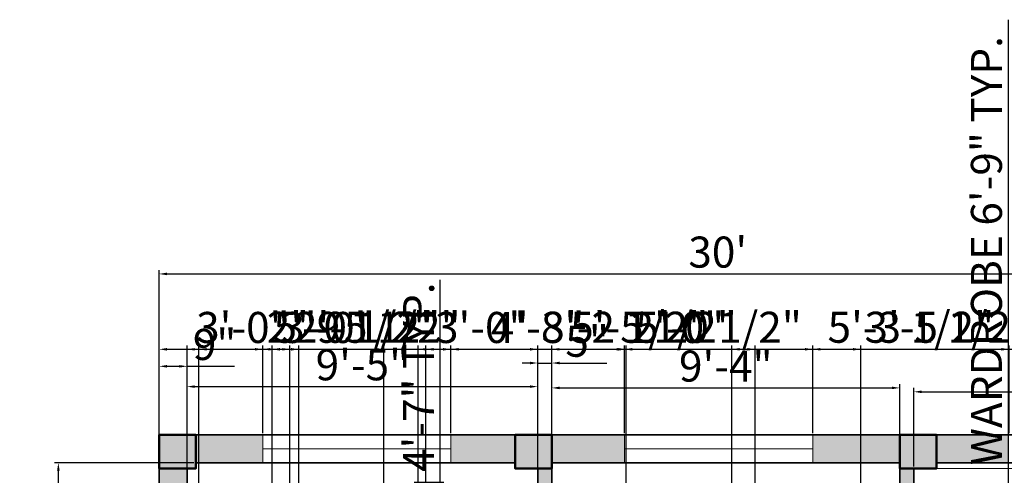
# Model space of a CAD drawing. Units: inches. Extents: x 2312 to 2808, y 1290 to 1909.
# Tile 4 of 5: x 2316 to 2633, y 1763 to 1909. Entities that reach past the tile are written whole.
import ezdxf

# ---------------------------------------------------------------- set-up
doc = ezdxf.new("R2010")
doc.units = ezdxf.units.IN
for name, color, linetype, lineweight in [('A-ANNO-DIMS', 2, 'Continuous', 18), ('A-COLS-PATT', 1, 'Continuous', 13), ('A-WALL-PATT', 150, 'Continuous', 13), ('COLUMN', 1, 'Continuous', 50), ('WALL', 7, 'Continuous', 35), ('WINDOW', 70, 'Continuous', 18)]:
    doc.layers.add(name, color=color, linetype=linetype, lineweight=lineweight)
doc.styles.get("Standard").update_dxf_attribs({"font": 'arial.ttf'})
doc.dimstyles.new('ISO-25', dxfattribs={"dimtxt": 10, "dimasz": 2.5, "dimexe": 1.25, "dimexo": 0.625, "dimtad": 1, "dimdec": 0, "dimlunit": 4, "dimtxsty": 'Standard', "dimcen": 2.5, "dimadec": 0, "dimazin": 0, "dimtfac": 1, "dimtdec": 0, "dimtmove": 0, "dimatfit": 3, "dimfxl": 1, "dimarcsym": 0})

# ---------------------------------------------------------------- blocks, each defined once
blk = doc.blocks.new('*D5')
at = {"layer": 'A-ANNO-DIMS', "color": 0, "lineweight": -2, "transparency": 16777216}
for p, q in [((2360.43, 1776.34), (2360.43, 1828.83)), ((2362.93, 1827.58), (2717.93, 1827.58)), ((2720.43, 1776.34), (2720.43, 1828.83))]:
    blk.add_line(p, q, dxfattribs=at)
at = {"layer": 'A-ANNO-DIMS', "color": 0, "transparency": 16777216}
for points in [[(2362.93, 1828), (2362.93, 1827.17), (2360.43, 1827.58)], [(2717.93, 1828), (2717.93, 1827.17), (2720.43, 1827.58)]]:
    blk.add_solid(points, dxfattribs=at)
at = {"layer": 'Defpoints', "color": 0, "transparency": 16777216}
for p in [(2720.43, 1827.58), (2360.43, 1775.72), (2720.43, 1775.72)]:
    blk.add_point(p, dxfattribs=at)
at = {"layer": 'A-ANNO-DIMS', "color": 0, "transparency": 16777216, "insert": (2540.43, 1833.32), "char_height": 10, "attachment_point": 5}
blk.add_mtext("30'", dxfattribs=at)
blk = doc.blocks.new('*D7')
at = {"layer": 'A-ANNO-DIMS', "color": 0, "lineweight": -2, "transparency": 16777216}
for p, q in [((2369.43, 1765.57), (2369.43, 1792.55)), ((2482.43, 1765.57), (2482.43, 1792.55)), ((2371.93, 1791.3), (2479.93, 1791.3))]:
    blk.add_line(p, q, dxfattribs=at)
at = {"layer": 'A-ANNO-DIMS', "color": 0, "transparency": 16777216}
for points in [[(2371.93, 1791.72), (2371.93, 1790.88), (2369.43, 1791.3)], [(2479.93, 1791.72), (2479.93, 1790.88), (2482.43, 1791.3)]]:
    blk.add_solid(points, dxfattribs=at)
at = {"layer": 'Defpoints', "color": 0, "transparency": 16777216}
for p in [(2482.43, 1791.3), (2369.43, 1764.94), (2482.43, 1764.94)]:
    blk.add_point(p, dxfattribs=at)
at = {"layer": 'A-ANNO-DIMS', "color": 0, "transparency": 16777216, "insert": (2425.93, 1797.03), "char_height": 10, "attachment_point": 5}
blk.add_mtext('9\'-5"', dxfattribs=at)
blk = doc.blocks.new('*D8')
at = {"layer": 'A-ANNO-DIMS', "color": 0, "lineweight": -2, "transparency": 16777216}
for p, q in [((2360.43, 1765.57), (2360.43, 1799.09)), ((2369.43, 1765.57), (2369.43, 1799.09)), ((2362.93, 1797.84), (2366.93, 1797.84)), ((2369.43, 1797.84), (2384.68, 1797.84))]:
    blk.add_line(p, q, dxfattribs=at)
at = {"layer": 'A-ANNO-DIMS', "color": 0, "transparency": 16777216}
for points in [[(2362.93, 1798.25), (2362.93, 1797.42), (2360.43, 1797.84)], [(2366.93, 1798.25), (2366.93, 1797.42), (2369.43, 1797.84)]]:
    blk.add_solid(points, dxfattribs=at)
at = {"layer": 'Defpoints', "color": 0, "transparency": 16777216}
for p in [(2369.43, 1797.84), (2360.43, 1764.94), (2369.43, 1764.94)]:
    blk.add_point(p, dxfattribs=at)
at = {"layer": 'A-ANNO-DIMS', "color": 0, "transparency": 16777216, "insert": (2378.31, 1803.57), "char_height": 10, "attachment_point": 5}
blk.add_mtext('9"', dxfattribs=at)
blk = doc.blocks.new('*D9')
at = {"layer": 'A-ANNO-DIMS', "color": 0, "lineweight": -2, "transparency": 16777216}
for p, q in [((2479.93, 1798.9), (2477.43, 1798.9)), ((2482.43, 1765.57), (2482.43, 1800.15)), ((2482.43, 1798.9), (2486.97, 1798.9)), ((2486.97, 1765.57), (2486.97, 1800.15)), ((2489.47, 1798.9), (2504.71, 1798.9))]:
    blk.add_line(p, q, dxfattribs=at)
at = {"layer": 'A-ANNO-DIMS', "color": 0, "transparency": 16777216}
for points in [[(2479.93, 1799.32), (2479.93, 1798.48), (2482.43, 1798.9)], [(2489.47, 1799.32), (2489.47, 1798.48), (2486.97, 1798.9)]]:
    blk.add_solid(points, dxfattribs=at)
at = {"layer": 'Defpoints', "color": 0, "transparency": 16777216}
for p in [(2486.97, 1798.9), (2482.43, 1764.94), (2486.97, 1764.94)]:
    blk.add_point(p, dxfattribs=at)
at = {"layer": 'A-ANNO-DIMS', "color": 0, "transparency": 16777216, "insert": (2498.34, 1804.61), "char_height": 10, "attachment_point": 5}
blk.add_mtext('5"', dxfattribs=at)
blk = doc.blocks.new('*D10')
at = {"layer": 'A-ANNO-DIMS', "color": 0, "lineweight": -2, "transparency": 16777216}
for p, q in [((2486.97, 1765.57), (2486.97, 1792.13)), ((2489.47, 1790.88), (2596.57, 1790.88)), ((2599.07, 1765.57), (2599.07, 1792.13))]:
    blk.add_line(p, q, dxfattribs=at)
at = {"layer": 'A-ANNO-DIMS', "color": 0, "transparency": 16777216}
for points in [[(2489.47, 1791.3), (2489.47, 1790.47), (2486.97, 1790.88)], [(2596.57, 1791.3), (2596.57, 1790.47), (2599.07, 1790.88)]]:
    blk.add_solid(points, dxfattribs=at)
at = {"layer": 'Defpoints', "color": 0, "transparency": 16777216}
for p in [(2599.07, 1790.88), (2486.97, 1764.94), (2599.07, 1764.94)]:
    blk.add_point(p, dxfattribs=at)
at = {"layer": 'A-ANNO-DIMS', "color": 0, "transparency": 16777216, "insert": (2543.02, 1796.61), "char_height": 10, "attachment_point": 5}
blk.add_mtext('9\'-4"', dxfattribs=at)
blk = doc.blocks.new('*D11')
at = {"layer": 'A-ANNO-DIMS', "color": 0, "lineweight": -2, "transparency": 16777216}
for p, q in [((2603.61, 1765.57), (2603.61, 1790.88)), ((2606.11, 1789.63), (2708.93, 1789.63)), ((2711.43, 1765.57), (2711.43, 1790.88))]:
    blk.add_line(p, q, dxfattribs=at)
at = {"layer": 'A-ANNO-DIMS', "color": 0, "transparency": 16777216}
for points in [[(2606.11, 1790.04), (2606.11, 1789.21), (2603.61, 1789.63)], [(2708.93, 1790.04), (2708.93, 1789.21), (2711.43, 1789.63)]]:
    blk.add_solid(points, dxfattribs=at)
at = {"layer": 'Defpoints', "color": 0, "transparency": 16777216}
for p in [(2711.43, 1789.63), (2603.61, 1764.94), (2711.43, 1764.94)]:
    blk.add_point(p, dxfattribs=at)
at = {"layer": 'A-ANNO-DIMS', "color": 0, "transparency": 16777216, "insert": (2657.52, 1795.36), "char_height": 10, "attachment_point": 5}
blk.add_mtext("9'", dxfattribs=at)
blk = doc.blocks.new('*D12')
at = {"layer": 'A-ANNO-DIMS', "color": 0, "lineweight": -2, "transparency": 16777216}
for p, q in [((2604.24, 1764.94), (2740.72, 1765.28)), ((2739.79, 1637.55), (2739.48, 1762.78)), ((2604.56, 1634.72), (2741.04, 1635.06))]:
    blk.add_line(p, q, dxfattribs=at)
at = {"layer": 'A-ANNO-DIMS', "color": 0, "transparency": 16777216}
for points in [[(2739.89, 1762.78), (2739.06, 1762.78), (2739.47, 1765.28)], [(2740.2, 1637.56), (2739.37, 1637.55), (2739.79, 1635.05)]]:
    blk.add_solid(points, dxfattribs=at)
at = {"layer": 'Defpoints', "color": 0, "transparency": 16777216}
for p in [(2603.61, 1764.94), (2739.47, 1765.28), (2603.93, 1634.72)]:
    blk.add_point(p, dxfattribs=at)
at = {"layer": 'A-ANNO-DIMS', "color": 0, "transparency": 16777216, "insert": (2745.36, 1700.18), "char_height": 10, "attachment_point": 5, "rotation": 270.1423}
blk.add_mtext('10\'-10"', dxfattribs=at)
blk = doc.blocks.new('*D21')
at = {"layer": 'A-ANNO-DIMS', "color": 0, "lineweight": -2, "transparency": 16777216}
for p, q in [((2371.65, 1766.72), (2326.71, 1766.72)), ((2327.96, 1637.22), (2327.96, 1764.22)), ((2371.65, 1634.72), (2326.71, 1634.72))]:
    blk.add_line(p, q, dxfattribs=at)
at = {"layer": 'A-ANNO-DIMS', "color": 0, "transparency": 16777216}
for points in [[(2327.54, 1764.22), (2328.38, 1764.22), (2327.96, 1766.72)], [(2327.54, 1637.22), (2328.38, 1637.22), (2327.96, 1634.72)]]:
    blk.add_solid(points, dxfattribs=at)
at = {"layer": 'Defpoints', "color": 0, "transparency": 16777216}
for p in [(2327.96, 1766.72), (2372.28, 1766.72), (2372.28, 1634.72)]:
    blk.add_point(p, dxfattribs=at)
at = {"layer": 'A-ANNO-DIMS', "color": 0, "transparency": 16777216, "insert": (2322.31, 1700.72), "char_height": 10, "attachment_point": 5, "rotation": 90}
blk.add_mtext("11'", dxfattribs=at)
blk = doc.blocks.new('*D30')
at = {"layer": 'A-ANNO-DIMS', "color": 0, "lineweight": -2, "transparency": 16777216}
for p, q in [((2450.95, 1760.54), (2450.95, 1825.65)), ((2442.63, 1760.54), (2452.2, 1760.54)), ((2450.95, 1707.96), (2450.95, 1758.04)), ((2442.63, 1705.46), (2452.2, 1705.46))]:
    blk.add_line(p, q, dxfattribs=at)
at = {"layer": 'A-ANNO-DIMS', "color": 0, "transparency": 16777216}
for points in [[(2450.54, 1758.04), (2451.37, 1758.04), (2450.95, 1760.54)], [(2450.54, 1707.96), (2451.37, 1707.96), (2450.95, 1705.46)]]:
    blk.add_solid(points, dxfattribs=at)
at = {"layer": 'Defpoints', "color": 0, "transparency": 16777216}
for p in [(2442, 1760.54), (2450.95, 1760.54), (2442, 1705.46)]:
    blk.add_point(p, dxfattribs=at)
at = {"layer": 'A-ANNO-DIMS', "color": 0, "transparency": 16777216, "insert": (2445.32, 1794.34), "char_height": 10, "attachment_point": 5, "rotation": 90}
blk.add_mtext('4\'-7" TYP.', dxfattribs=at)
blk = doc.blocks.new('*D31')
at = {"layer": 'A-ANNO-DIMS', "color": 0, "lineweight": -2, "transparency": 16777216}
for p, q in [((2634.1, 1758.19), (2634.1, 1909.46)), ((2622.58, 1758.19), (2635.35, 1758.19)), ((2634.1, 1679.72), (2634.1, 1755.69)), ((2622.58, 1677.22), (2635.35, 1677.22))]:
    blk.add_line(p, q, dxfattribs=at)
at = {"layer": 'A-ANNO-DIMS', "color": 0, "transparency": 16777216}
for points in [[(2633.68, 1755.69), (2634.51, 1755.69), (2634.1, 1758.19)], [(2633.68, 1679.72), (2634.51, 1679.72), (2634.1, 1677.22)]]:
    blk.add_solid(points, dxfattribs=at)
at = {"layer": 'Defpoints', "color": 0, "transparency": 16777216}
for p in [(2621.95, 1758.19), (2634.1, 1758.19), (2621.95, 1677.22)]:
    blk.add_point(p, dxfattribs=at)
at = {"layer": 'A-ANNO-DIMS', "color": 0, "transparency": 16777216, "insert": (2628.3, 1835.07), "char_height": 10, "attachment_point": 5, "rotation": 90}
blk.add_mtext('WARDROBE 6\'-9" TYP.', dxfattribs=at)
blk = doc.blocks.new('*D41')
at = {"layer": 'A-ANNO-DIMS', "color": 0, "lineweight": -2, "transparency": 16777216}
for p, q in [((2443.93, 1546.83), (2443.93, 1804.57)), ((2446.43, 1803.32), (2479.93, 1803.32)), ((2482.43, 1510.12), (2482.43, 1804.57)), ((2482.43, 1803.32), (2536.06, 1803.32))]:
    blk.add_line(p, q, dxfattribs=at)
at = {"layer": 'A-ANNO-DIMS', "color": 0, "transparency": 16777216}
for points in [[(2446.43, 1803.73), (2446.43, 1802.9), (2443.93, 1803.32)], [(2479.93, 1803.73), (2479.93, 1802.9), (2482.43, 1803.32)]]:
    blk.add_solid(points, dxfattribs=at)
at = {"layer": 'Defpoints', "color": 0, "transparency": 16777216}
for p in [(2482.43, 1803.32), (2443.93, 1546.2), (2482.43, 1509.49)]:
    blk.add_point(p, dxfattribs=at)
at = {"layer": 'A-ANNO-DIMS', "color": 0, "transparency": 16777216, "insert": (2510.5, 1809.12), "char_height": 10, "attachment_point": 5}
blk.add_mtext('3\'-2 1/2"', dxfattribs=at)
blk = doc.blocks.new('*D43')
at = {"layer": 'A-ANNO-DIMS', "color": 0, "lineweight": -2, "transparency": 16777216}
for p, q in [((2486.93, 1401.34), (2486.93, 1804.57)), ((2489.43, 1803.32), (2508.43, 1803.32)), ((2510.93, 1401.34), (2510.93, 1804.57)), ((2510.93, 1803.32), (2541.44, 1803.32))]:
    blk.add_line(p, q, dxfattribs=at)
at = {"layer": 'A-ANNO-DIMS', "color": 0, "transparency": 16777216}
for points in [[(2489.43, 1803.73), (2489.43, 1802.9), (2486.93, 1803.32)], [(2508.43, 1803.73), (2508.43, 1802.9), (2510.93, 1803.32)]]:
    blk.add_solid(points, dxfattribs=at)
at = {"layer": 'Defpoints', "color": 0, "transparency": 16777216}
for p in [(2510.93, 1803.32), (2486.93, 1400.72), (2510.93, 1400.72)]:
    blk.add_point(p, dxfattribs=at)
at = {"layer": 'A-ANNO-DIMS', "color": 0, "transparency": 16777216, "insert": (2527.44, 1809.05), "char_height": 10, "attachment_point": 5}
blk.add_mtext('2\'-0"', dxfattribs=at)
blk = doc.blocks.new('*D44')
at = {"layer": 'A-ANNO-DIMS', "color": 0, "lineweight": -2, "transparency": 16777216}
for p, q in [((2360.43, 1776.34), (2360.43, 1804.57)), ((2362.93, 1803.32), (2391.3, 1803.32)), ((2393.8, 1776.34), (2393.8, 1804.57)), ((2393.8, 1803.32), (2447.6, 1803.32))]:
    blk.add_line(p, q, dxfattribs=at)
at = {"layer": 'A-ANNO-DIMS', "color": 0, "transparency": 16777216}
for points in [[(2362.93, 1803.73), (2362.93, 1802.9), (2360.43, 1803.32)], [(2391.3, 1803.73), (2391.3, 1802.9), (2393.8, 1803.32)]]:
    blk.add_solid(points, dxfattribs=at)
at = {"layer": 'Defpoints', "color": 0, "transparency": 16777216}
for p in [(2393.8, 1803.32), (2360.43, 1775.72), (2393.8, 1775.72)]:
    blk.add_point(p, dxfattribs=at)
at = {"layer": 'A-ANNO-DIMS', "color": 0, "transparency": 16777216, "insert": (2421.95, 1809.11), "char_height": 10, "attachment_point": 5}
blk.add_mtext('2\'-9 1/2"', dxfattribs=at)
blk = doc.blocks.new('*D45')
at = {"layer": 'A-ANNO-DIMS', "color": 0, "lineweight": -2, "transparency": 16777216}
for p, q in [((2393.8, 1776.34), (2393.8, 1804.57)), ((2396.3, 1803.32), (2451.95, 1803.32)), ((2454.45, 1776.34), (2454.45, 1804.57))]:
    blk.add_line(p, q, dxfattribs=at)
at = {"layer": 'A-ANNO-DIMS', "color": 0, "transparency": 16777216}
for points in [[(2396.3, 1803.73), (2396.3, 1802.9), (2393.8, 1803.32)], [(2451.95, 1803.73), (2451.95, 1802.9), (2454.45, 1803.32)]]:
    blk.add_solid(points, dxfattribs=at)
at = {"layer": 'Defpoints', "color": 0, "transparency": 16777216}
for p in [(2454.45, 1803.32), (2393.8, 1775.72), (2454.45, 1775.72)]:
    blk.add_point(p, dxfattribs=at)
at = {"layer": 'A-ANNO-DIMS', "color": 0, "transparency": 16777216, "insert": (2424.12, 1809.11), "char_height": 10, "attachment_point": 5}
blk.add_mtext('5\'-0 1/2"', dxfattribs=at)
blk = doc.blocks.new('*D46')
at = {"layer": 'A-ANNO-DIMS', "color": 0, "lineweight": -2, "transparency": 16777216}
for p, q in [((2454.45, 1776.34), (2454.45, 1804.57)), ((2456.95, 1803.32), (2507.86, 1803.32)), ((2510.36, 1776.34), (2510.36, 1804.57))]:
    blk.add_line(p, q, dxfattribs=at)
at = {"layer": 'A-ANNO-DIMS', "color": 0, "transparency": 16777216}
for points in [[(2456.95, 1803.73), (2456.95, 1802.9), (2454.45, 1803.32)], [(2507.86, 1803.73), (2507.86, 1802.9), (2510.36, 1803.32)]]:
    blk.add_solid(points, dxfattribs=at)
at = {"layer": 'Defpoints', "color": 0, "transparency": 16777216}
for p in [(2510.36, 1803.32), (2454.45, 1775.72), (2510.36, 1775.72)]:
    blk.add_point(p, dxfattribs=at)
at = {"layer": 'A-ANNO-DIMS', "color": 0, "transparency": 16777216, "insert": (2482.41, 1809.05), "char_height": 10, "attachment_point": 5}
blk.add_mtext('4\'-8"', dxfattribs=at)
blk = doc.blocks.new('*D47')
at = {"layer": 'A-ANNO-DIMS', "color": 0, "lineweight": -2, "transparency": 16777216}
for p, q in [((2510.36, 1776.34), (2510.36, 1804.57)), ((2512.86, 1803.32), (2568.52, 1803.32)), ((2571.02, 1776.34), (2571.02, 1804.57))]:
    blk.add_line(p, q, dxfattribs=at)
at = {"layer": 'A-ANNO-DIMS', "color": 0, "transparency": 16777216}
for points in [[(2512.86, 1803.73), (2512.86, 1802.9), (2510.36, 1803.32)], [(2568.52, 1803.73), (2568.52, 1802.9), (2571.02, 1803.32)]]:
    blk.add_solid(points, dxfattribs=at)
at = {"layer": 'Defpoints', "color": 0, "transparency": 16777216}
for p in [(2571.02, 1803.32), (2510.36, 1775.72), (2571.02, 1775.72)]:
    blk.add_point(p, dxfattribs=at)
at = {"layer": 'A-ANNO-DIMS', "color": 0, "transparency": 16777216, "insert": (2540.69, 1809.11), "char_height": 10, "attachment_point": 5}
blk.add_mtext('5\'-0 1/2"', dxfattribs=at)
blk = doc.blocks.new('*D48')
at = {"layer": 'A-ANNO-DIMS', "color": 0, "lineweight": -2, "transparency": 16777216}
for p, q in [((2571.02, 1776.34), (2571.02, 1804.57)), ((2573.52, 1803.32), (2631.81, 1803.32)), ((2634.31, 1776.34), (2634.31, 1804.57))]:
    blk.add_line(p, q, dxfattribs=at)
at = {"layer": 'A-ANNO-DIMS', "color": 0, "transparency": 16777216}
for points in [[(2573.52, 1803.73), (2573.52, 1802.9), (2571.02, 1803.32)], [(2631.81, 1803.73), (2631.81, 1802.9), (2634.31, 1803.32)]]:
    blk.add_solid(points, dxfattribs=at)
at = {"layer": 'Defpoints', "color": 0, "transparency": 16777216}
for p in [(2634.31, 1803.32), (2571.02, 1775.72), (2634.31, 1775.72)]:
    blk.add_point(p, dxfattribs=at)
at = {"layer": 'A-ANNO-DIMS', "color": 0, "transparency": 16777216, "insert": (2602.66, 1809.12), "char_height": 10, "attachment_point": 5}
blk.add_mtext('5\'-3 1/2"', dxfattribs=at)
blk = doc.blocks.new('*D50')
at = {"layer": 'A-ANNO-DIMS', "color": 0, "lineweight": -2, "transparency": 16777216}
for p, q in [((2446.36, 1635.34), (2446.36, 1804.57)), ((2448.86, 1803.32), (2479.93, 1803.32)), ((2482.43, 1635.34), (2482.43, 1804.57))]:
    blk.add_line(p, q, dxfattribs=at)
at = {"layer": 'A-ANNO-DIMS', "color": 0, "transparency": 16777216}
for points in [[(2448.86, 1803.73), (2448.86, 1802.9), (2446.36, 1803.32)], [(2479.93, 1803.73), (2479.93, 1802.9), (2482.43, 1803.32)]]:
    blk.add_solid(points, dxfattribs=at)
at = {"layer": 'Defpoints', "color": 0, "transparency": 16777216}
for p in [(2482.43, 1803.32), (2446.36, 1634.72), (2482.43, 1634.72)]:
    blk.add_point(p, dxfattribs=at)
at = {"layer": 'A-ANNO-DIMS', "color": 0, "transparency": 16777216, "insert": (2464.4, 1809.05), "char_height": 10, "attachment_point": 5}
blk.add_mtext('3\'-0"', dxfattribs=at)
blk = doc.blocks.new('*D53')
at = {"layer": 'A-ANNO-DIMS', "color": 0, "lineweight": -2, "transparency": 16777216}
for p, q in [((2369.43, 1543.69), (2369.43, 1804.57)), ((2371.93, 1803.32), (2402.93, 1803.32)), ((2405.43, 1539.84), (2405.43, 1804.57))]:
    blk.add_line(p, q, dxfattribs=at)
at = {"layer": 'A-ANNO-DIMS', "color": 0, "transparency": 16777216}
for points in [[(2371.93, 1803.73), (2371.93, 1802.9), (2369.43, 1803.32)], [(2402.93, 1803.73), (2402.93, 1802.9), (2405.43, 1803.32)]]:
    blk.add_solid(points, dxfattribs=at)
at = {"layer": 'Defpoints', "color": 0, "transparency": 16777216}
for p in [(2405.43, 1803.32), (2369.43, 1543.07), (2405.43, 1539.22)]:
    blk.add_point(p, dxfattribs=at)
at = {"layer": 'A-ANNO-DIMS', "color": 0, "transparency": 16777216, "insert": (2387.43, 1809.05), "char_height": 10, "attachment_point": 5}
blk.add_mtext('3\'-0"', dxfattribs=at)
blk = doc.blocks.new('*D54')
at = {"layer": 'A-ANNO-DIMS', "color": 0, "lineweight": -2, "transparency": 16777216}
for p, q in [((2545.01, 1581.25), (2545.01, 1804.57)), ((2547.51, 1803.32), (2583.99, 1803.32)), ((2586.49, 1581.25), (2586.49, 1804.57)), ((2586.49, 1803.32), (2640.12, 1803.32))]:
    blk.add_line(p, q, dxfattribs=at)
at = {"layer": 'A-ANNO-DIMS', "color": 0, "transparency": 16777216}
for points in [[(2547.51, 1803.73), (2547.51, 1802.9), (2545.01, 1803.32)], [(2583.99, 1803.73), (2583.99, 1802.9), (2586.49, 1803.32)]]:
    blk.add_solid(points, dxfattribs=at)
at = {"layer": 'Defpoints', "color": 0, "transparency": 16777216}
for p in [(2586.49, 1803.32), (2545.01, 1580.62), (2586.49, 1580.62)]:
    blk.add_point(p, dxfattribs=at)
at = {"layer": 'A-ANNO-DIMS', "color": 0, "transparency": 16777216, "insert": (2614.56, 1809.12), "char_height": 10, "attachment_point": 5}
blk.add_mtext('3\'-5 1/2"', dxfattribs=at)
blk = doc.blocks.new('*D62')
at = {"layer": 'A-ANNO-DIMS', "color": 0, "lineweight": -2, "transparency": 16777216}
for p, q in [((2396.83, 1508.42), (2396.83, 1804.57)), ((2399.33, 1803.32), (2430.33, 1803.32)), ((2432.83, 1508.42), (2432.83, 1804.57))]:
    blk.add_line(p, q, dxfattribs=at)
at = {"layer": 'A-ANNO-DIMS', "color": 0, "transparency": 16777216}
for points in [[(2399.33, 1803.73), (2399.33, 1802.9), (2396.83, 1803.32)], [(2430.33, 1803.73), (2430.33, 1802.9), (2432.83, 1803.32)]]:
    blk.add_solid(points, dxfattribs=at)
at = {"layer": 'Defpoints', "color": 0, "transparency": 16777216}
for p in [(2432.83, 1803.32), (2396.83, 1507.8), (2432.83, 1507.8)]:
    blk.add_point(p, dxfattribs=at)
at = {"layer": 'A-ANNO-DIMS', "color": 0, "transparency": 16777216, "insert": (2414.83, 1809.05), "char_height": 10, "attachment_point": 5}
blk.add_mtext('3\'-0"', dxfattribs=at)
blk = doc.blocks.new('*D67')
at = {"layer": 'A-ANNO-DIMS', "color": 0, "lineweight": -2, "transparency": 16777216}
for p, q in [((2486.93, 1499.34), (2486.93, 1804.57)), ((2489.43, 1803.32), (2550.01, 1803.32)), ((2552.51, 1499.34), (2552.51, 1804.57))]:
    blk.add_line(p, q, dxfattribs=at)
at = {"layer": 'A-ANNO-DIMS', "color": 0, "transparency": 16777216}
for points in [[(2489.43, 1803.73), (2489.43, 1802.9), (2486.93, 1803.32)], [(2550.01, 1803.73), (2550.01, 1802.9), (2552.51, 1803.32)]]:
    blk.add_solid(points, dxfattribs=at)
at = {"layer": 'Defpoints', "color": 0, "transparency": 16777216}
for p in [(2552.51, 1803.32), (2486.93, 1498.72), (2552.51, 1498.72)]:
    blk.add_point(p, dxfattribs=at)
at = {"layer": 'A-ANNO-DIMS', "color": 0, "transparency": 16777216, "insert": (2519.72, 1809.11), "char_height": 10, "attachment_point": 5}
blk.add_mtext('5\'-5 1/2"', dxfattribs=at)
blk = doc.blocks.new('*D73')
at = {"layer": 'A-ANNO-DIMS', "color": 0, "lineweight": -2, "transparency": 16777216}
for p, q in [((2373.27, 1609.07), (2373.27, 1804.57)), ((2375.77, 1803.32), (2400.08, 1803.32)), ((2402.58, 1609.07), (2402.58, 1804.57)), ((2402.58, 1803.32), (2456.39, 1803.32))]:
    blk.add_line(p, q, dxfattribs=at)
at = {"layer": 'A-ANNO-DIMS', "color": 0, "transparency": 16777216}
for points in [[(2375.77, 1803.73), (2375.77, 1802.9), (2373.27, 1803.32)], [(2400.08, 1803.73), (2400.08, 1802.9), (2402.58, 1803.32)]]:
    blk.add_solid(points, dxfattribs=at)
at = {"layer": 'Defpoints', "color": 0, "transparency": 16777216}
for p in [(2402.58, 1803.32), (2373.27, 1608.44), (2402.58, 1608.44)]:
    blk.add_point(p, dxfattribs=at)
at = {"layer": 'A-ANNO-DIMS', "color": 0, "transparency": 16777216, "insert": (2430.74, 1809.11), "char_height": 10, "attachment_point": 5}
blk.add_mtext('2\'-5 1/2"', dxfattribs=at)

msp = doc.modelspace()

# ---------------------------------------------------------------- hatches: boundary and pattern name
at = {"layer": 'A-COLS-PATT'}
h = msp.add_hatch(color=256, dxfattribs=at)
h.dxf.hatch_style = 1
h.paths.add_polyline_path([(2372.28, 1775.72), (2360.43, 1775.72), (2360.43, 1764.94), (2372.28, 1764.94)])
h.paths.add_polyline_path([(2486.97, 1775.72), (2475.12, 1775.72), (2475.12, 1764.94), (2486.93, 1764.94), (2486.93, 1766.72)])
h.paths.add_polyline_path([(2610.92, 1775.72), (2599.07, 1775.72), (2599.07, 1766.72), (2599.11, 1766.72), (2599.11, 1764.94), (2610.92, 1764.94)])
h.paths.add_polyline_path([(2720.43, 1775.72), (2708.59, 1775.72), (2708.59, 1764.94), (2720.43, 1764.94)])
h.paths.add_polyline_path([(2723.28, 1640.11), (2711.43, 1640.11), (2711.43, 1629.34), (2723.28, 1629.34)])
h.paths.add_polyline_path([(2603.61, 1640.99), (2592.09, 1640.99), (2592.09, 1630.22), (2603.93, 1630.22), (2603.93, 1634.72), (2603.61, 1634.72)])
h.paths.add_polyline_path([(2494.28, 1640.99), (2482.43, 1640.99), (2482.43, 1630.22), (2494.28, 1630.22)])
h.paths.add_polyline_path([(2372.28, 1640.99), (2360.43, 1640.99), (2360.43, 1630.22), (2372.28, 1630.22)])
h.paths.add_polyline_path([(2372.28, 1509.49), (2360.43, 1509.49), (2360.43, 1498.72), (2372.28, 1498.72)])
h.paths.add_polyline_path([(2494.28, 1509.49), (2482.43, 1509.49), (2482.43, 1498.72), (2494.28, 1498.72)])
h.paths.add_polyline_path([(2603.93, 1509.49), (2592.09, 1509.49), (2592.09, 1498.72), (2603.93, 1498.72)])
h.paths.add_polyline_path([(2723.28, 1509.26), (2711.43, 1509.26), (2711.43, 1498.48), (2723.28, 1498.48)])
h.paths.add_polyline_path([(2720.43, 1378.49), (2708.59, 1378.49), (2708.59, 1367.72), (2720.43, 1367.72)])
h.paths.add_polyline_path([(2610.2, 1378.49), (2598.36, 1378.49), (2598.36, 1367.72), (2610.2, 1367.72)])
h.paths.add_polyline_path([(2486.94, 1376.72), (2486.93, 1376.72), (2486.93, 1378.49), (2475.1, 1378.49), (2475.1, 1367.72), (2486.94, 1367.72)])
h.paths.add_polyline_path([(2372.28, 1378.49), (2360.43, 1378.49), (2360.43, 1367.72), (2372.28, 1367.72)])
at = {"layer": 'A-WALL-PATT'}
h = msp.add_hatch(color=256, dxfattribs=at)
h.dxf.hatch_style = 1
h.paths.add_polyline_path([(2369.43, 1764.94), (2360.43, 1764.94), (2360.43, 1640.99), (2369.43, 1640.99)])
h.paths.add_polyline_path([(2720.43, 1764.94), (2711.43, 1764.94), (2711.43, 1640.11), (2720.43, 1640.11)])
h.paths.add_polyline_path([(2552.09, 1634.72), (2494.28, 1634.72), (2494.28, 1630.22), (2552.09, 1630.22)])
h.paths.add_polyline_path([(2446.36, 1634.72), (2372.28, 1634.72), (2372.28, 1630.22), (2405.43, 1630.22), (2439.43, 1630.22), (2446.36, 1630.22)])
h.paths.add_polyline_path([(2443.93, 1630.22), (2439.43, 1630.22), (2439.43, 1596.05), (2443.93, 1596.05)])
h.paths.add_polyline_path([(2486.93, 1630.22), (2482.43, 1630.22), (2482.43, 1509.49), (2486.93, 1509.49)])
h.paths.add_polyline_path([(2443.93, 1546.2), (2439.43, 1546.2), (2439.43, 1503.22), (2372.28, 1503.22), (2372.28, 1498.72), (2443.93, 1498.72)])
h.paths.add_polyline_path([(2555.45, 1503.22), (2494.28, 1503.22), (2494.28, 1498.72), (2555.45, 1498.72)])
h.paths.add_polyline_path([(2711.43, 1503.22), (2639.88, 1503.22), (2639.88, 1498.72), (2711.43, 1498.72)])
h.paths.add_polyline_path([(2646.41, 1564.72), (2711.43, 1564.72), (2711.43, 1569.22), (2646.41, 1569.22), (2646.41, 1597.21), (2641.91, 1597.21), (2641.91, 1564.72), (2641.91, 1536.48), (2646.41, 1536.48)])
h.paths.add_polyline_path([(2720.43, 1498.48), (2711.43, 1498.48), (2711.43, 1378.49), (2720.43, 1378.49)])
h.paths.add_polyline_path([(2369.43, 1498.72), (2360.43, 1498.72), (2360.43, 1378.49), (2369.43, 1378.49)])
h.paths.add_polyline_path([(2486.93, 1498.72), (2482.43, 1498.72), (2482.43, 1378.49), (2486.93, 1378.49)])
h.paths.add_polyline_path([(2603.93, 1498.72), (2599.11, 1498.72), (2599.11, 1378.49), (2603.93, 1378.49)])
h.paths.add_polyline_path([(2510.36, 1766.72), (2510.36, 1775.72), (2486.97, 1775.72), (2486.97, 1766.72)])
h.paths.add_polyline_path([(2571.02, 1775.72), (2571.02, 1766.72), (2599.07, 1766.72), (2599.07, 1775.72)])
h.paths.add_polyline_path([(2393.8, 1766.72), (2393.8, 1775.72), (2372.28, 1775.72), (2372.28, 1766.72)])
h.paths.add_polyline_path([(2454.45, 1775.72), (2454.45, 1766.72), (2475.12, 1766.72), (2475.12, 1775.72)])
h.paths.add_polyline_path([(2694.96, 1775.72), (2694.96, 1766.72), (2708.59, 1766.72), (2708.59, 1775.72)])
h.paths.add_polyline_path([(2634.31, 1766.72), (2634.31, 1775.72), (2610.92, 1775.72), (2610.92, 1766.72)])
h.paths.add_polyline_path([(2392.25, 1367.72), (2392.25, 1376.72), (2372.28, 1376.72), (2372.28, 1367.72)])
h.paths.add_polyline_path([(2452.9, 1376.72), (2452.9, 1367.72), (2475.1, 1367.72), (2475.1, 1376.72)])
h.paths.add_polyline_path([(2508.56, 1376.72), (2508.56, 1367.72), (2558.63, 1367.72), (2558.63, 1370.65), (2558.63, 1376.72)])
h.paths.add_polyline_path([(2488.96, 1367.72), (2488.96, 1376.72), (2486.94, 1376.72), (2486.94, 1367.72)])
h.paths.add_polyline_path([(2634.6, 1367.72), (2634.6, 1376.72), (2610.2, 1376.72), (2610.2, 1367.72)])
h.paths.add_polyline_path([(2695.25, 1376.72), (2695.25, 1367.72), (2708.59, 1367.72), (2708.59, 1376.72)])
h.paths.add_polyline_path([(2360.43, 1590.4), (2369.43, 1590.4), (2369.43, 1630.22), (2360.43, 1630.22)])
h.paths.add_polyline_path([(2369.43, 1543.07), (2360.43, 1543.07), (2360.43, 1509.49), (2369.43, 1509.49)])
h.paths.add_polyline_path([(2720.43, 1531.67), (2711.43, 1531.67), (2711.43, 1509.26), (2720.43, 1509.26)])
h.paths.add_polyline_path([(2720.43, 1572.68), (2711.43, 1572.68), (2711.43, 1558.71), (2720.43, 1558.71)])
h.paths.add_polyline_path([(2711.43, 1599.72), (2720.43, 1599.72), (2720.43, 1629.34), (2711.43, 1629.34)])
h = msp.add_hatch(color=256, dxfattribs=at)
h.dxf.hatch_style = 1
h.paths.add_polyline_path([(2486.93, 1764.94), (2482.43, 1764.94), (2482.43, 1640.99), (2486.93, 1640.99)])
h.paths.add_polyline_path([(2603.61, 1764.94), (2599.11, 1764.94), (2599.11, 1640.99), (2603.61, 1640.99)])

# ---------------------------------------------------------------- linework, layer by layer
at = {"layer": 'COLUMN'}
for points in [[(2360.43, 1775.72), (2372.28, 1775.72), (2372.28, 1764.94), (2360.43, 1764.94)], [(2475.12, 1775.72), (2486.97, 1775.72), (2486.97, 1764.94), (2475.12, 1764.94)], [(2599.07, 1775.72), (2610.92, 1775.72), (2610.92, 1764.94), (2599.07, 1764.94)]]:
    msp.add_lwpolyline(points, close=True, dxfattribs=at)
at = {"layer": 'WALL'}
for p, q in [((2360.43, 1775.72), (2720.43, 1775.72)), ((2360.43, 1367.72), (2360.43, 1775.72)), ((2372.28, 1766.72), (2475.12, 1766.72)), ((2482.43, 1764.94), (2482.43, 1634.72)), ((2486.93, 1766.72), (2486.93, 1640.99)), ((2486.93, 1766.72), (2599.11, 1766.72)), ((2599.11, 1766.72), (2599.11, 1640.99)), ((2603.61, 1764.94), (2603.61, 1634.72))]:
    msp.add_line(p, q, dxfattribs=at)
for points in [[(2720.43, 1498.48), (2720.43, 1367.72), (2360.43, 1367.72), (2360.43, 1775.72), (2720.43, 1775.72), (2720.43, 1640.11)], [(2369.43, 1640.99), (2369.43, 1764.94)], [(2372.28, 1766.72), (2475.12, 1766.72)], [(2486.93, 1766.72), (2599.11, 1766.72)], [(2610.92, 1766.72), (2708.59, 1766.72)]]:
    msp.add_lwpolyline(points, dxfattribs=at)
at = {"layer": 'WINDOW'}
for p, q in [((2393.8, 1771.22), (2454.45, 1771.22)), ((2510.36, 1771.22), (2571.02, 1771.22))]:
    msp.add_line(p, q, dxfattribs=at)
for points in [[(2393.8, 1775.72), (2454.45, 1775.72), (2454.45, 1766.72), (2393.8, 1766.72)], [(2510.36, 1775.72), (2571.02, 1775.72), (2571.02, 1766.72), (2510.36, 1766.72)]]:
    msp.add_lwpolyline(points, close=True, dxfattribs=at)

# ---------------------------------------------------------------- dimensions: what is measured, and where the dimension line sits
at = {"layer": 'A-ANNO-DIMS'}
for base, p1, p2, text, picture, middle in [((2634.1, 1758.19), (2621.95, 1677.22), (2621.95, 1758.19), 'WARDROBE <> TYP.', '*D31', (2628.3, 1835.07)), ((2450.95, 1760.54), (2442, 1705.46), (2442, 1760.54), '<> TYP.', '*D30', (2445.32, 1794.34))]:
    dim = msp.add_linear_dim(base=base, p1=p1, p2=p2, angle=90, text=text, dimstyle='ISO-25', override={"dimdec": 1, "dimlfac": 1, "dimrnd": 0, "dimzin": 1, "dimdsep": 46, "dimlunit": 4, "dimfrac": 2}, dxfattribs=at)
    dim.commit()
    dim.dimension.update_dxf_attribs({"geometry": picture, "text_midpoint": middle})
for base, p1, p2, override, picture, middle in [((2720.43, 1827.58), (2360.43, 1775.72), (2720.43, 1775.72), {"dimclrd": 0, "dimclre": 0, "dimclrt": 0}, '*D5', (2540.43, 1833.32)), ((2393.8, 1803.32), (2360.43, 1775.72), (2393.8, 1775.72), {"dimdec": 1, "dimlfac": 1, "dimrnd": 0, "dimzin": 1, "dimdsep": 46, "dimlunit": 4, "dimfrac": 2}, '*D44', (2421.95, 1809.11)), ((2402.58, 1803.32), (2373.27, 1608.44), (2402.58, 1608.44), {"dimdec": 1, "dimlfac": 1, "dimrnd": 0, "dimzin": 1, "dimdsep": 46, "dimlunit": 4, "dimfrac": 2}, '*D73', (2430.74, 1809.11)), ((2454.4493, 1803.3175), (2393.7969, 1775.7175), (2454.4493, 1775.7175), {"dimdec": 1, "dimlfac": 1, "dimrnd": 0, "dimzin": 1, "dimdsep": 46, "dimlunit": 4, "dimfrac": 2}, '*D45', (2424.1231, 1809.113)), ((2482.43, 1803.32), (2443.93, 1546.2), (2482.43, 1509.49), {"dimdec": 1, "dimlfac": 1, "dimrnd": 0, "dimzin": 1, "dimdsep": 46, "dimlunit": 4, "dimfrac": 2}, '*D41', (2510.5, 1809.12)), ((2552.51, 1803.32), (2486.93, 1498.72), (2552.51, 1498.72), {"dimdec": 1, "dimlfac": 1, "dimrnd": 0, "dimzin": 1, "dimdsep": 46, "dimlunit": 4, "dimfrac": 2}, '*D67', (2519.72, 1809.11)), ((2571.02, 1803.32), (2510.36, 1775.72), (2571.02, 1775.72), {"dimdec": 1, "dimlfac": 1, "dimrnd": 0, "dimzin": 1, "dimdsep": 46, "dimlunit": 4, "dimfrac": 2}, '*D47', (2540.69, 1809.11)), ((2586.49, 1803.32), (2545.01, 1580.62), (2586.49, 1580.62), {"dimdec": 1, "dimlfac": 1, "dimrnd": 0, "dimzin": 1, "dimdsep": 46, "dimlunit": 4, "dimfrac": 2}, '*D54', (2614.56, 1809.12)), ((2634.31, 1803.32), (2571.02, 1775.72), (2634.31, 1775.72), {"dimdec": 1, "dimlfac": 1, "dimrnd": 0, "dimzin": 1, "dimdsep": 46, "dimlunit": 4, "dimfrac": 2}, '*D48', (2602.66, 1809.12)), ((2405.43, 1803.32), (2369.43, 1543.07), (2405.43, 1539.22), {"dimdec": 1, "dimlfac": 1, "dimrnd": 0, "dimzin": 1, "dimdsep": 46, "dimlunit": 4, "dimfrac": 2}, '*D53', (2387.43, 1809.05)), ((2432.83, 1803.32), (2396.83, 1507.8), (2432.83, 1507.8), {"dimdec": 1, "dimlfac": 1, "dimrnd": 0, "dimzin": 1, "dimdsep": 46, "dimlunit": 4, "dimfrac": 2}, '*D62', (2414.83, 1809.05)), ((2482.43, 1803.32), (2446.36, 1634.72), (2482.43, 1634.72), {"dimdec": 1, "dimlfac": 1, "dimrnd": 0, "dimzin": 1, "dimdsep": 46, "dimlunit": 4, "dimfrac": 2}, '*D50', (2464.4, 1809.05)), ((2510.36, 1803.32), (2454.45, 1775.72), (2510.36, 1775.72), {"dimdec": 1, "dimlfac": 1, "dimrnd": 0, "dimzin": 1, "dimdsep": 46, "dimlunit": 4, "dimfrac": 2}, '*D46', (2482.41, 1809.05)), ((2510.93, 1803.32), (2486.93, 1400.72), (2510.93, 1400.72), {"dimdec": 1, "dimlfac": 1, "dimrnd": 0, "dimzin": 1, "dimdsep": 46, "dimlunit": 4, "dimfrac": 2}, '*D43', (2527.44, 1809.05)), ((2369.43, 1797.84), (2360.43, 1764.94), (2369.43, 1764.94), {"dimclrd": 0, "dimclre": 0, "dimclrt": 0}, '*D8', (2378.31, 1803.57)), ((2486.97, 1798.9), (2482.43, 1764.94), (2486.97, 1764.94), {"dimclrd": 0, "dimclre": 0, "dimclrt": 0}, '*D9', (2498.34, 1804.61)), ((2482.43, 1791.3), (2369.43, 1764.94), (2482.43, 1764.94), {"dimclrd": 0, "dimclre": 0, "dimclrt": 0}, '*D7', (2425.93, 1797.03)), ((2599.07, 1790.88), (2486.97, 1764.94), (2599.07, 1764.94), {"dimclrd": 0, "dimclre": 0, "dimclrt": 0}, '*D10', (2543.02, 1796.61)), ((2711.43, 1789.63), (2603.61, 1764.94), (2711.43, 1764.94), {"dimclrd": 0, "dimclre": 0, "dimclrt": 0}, '*D11', (2657.52, 1795.36))]:
    dim = msp.add_linear_dim(base=base, p1=p1, p2=p2, dimstyle='ISO-25', override=override, dxfattribs=at)
    dim.commit()
    dim.dimension.update_dxf_attribs({"geometry": picture, "text_midpoint": middle})
dim = msp.add_linear_dim(base=(2327.96, 1766.72), p1=(2372.28, 1634.72), p2=(2372.28, 1766.72), angle=90, dimstyle='ISO-25', override={"dimclrd": 0, "dimclre": 0, "dimclrt": 0}, dxfattribs=at)
dim.commit()
dim.dimension.update_dxf_attribs({"geometry": '*D21', "text_midpoint": (2322.31, 1700.72)})
dim = msp.add_aligned_dim(p1=(2603.93, 1634.72), p2=(2603.61, 1764.94), distance=-135.86, dimstyle='ISO-25', override={"dimclrd": 0, "dimclre": 0, "dimclrt": 0}, dxfattribs=at)
dim.commit()
dim.dimension.update_dxf_attribs({"geometry": '*D12', "text_midpoint": (2745.36, 1700.18)})

doc.saveas('drawing.dxf')
